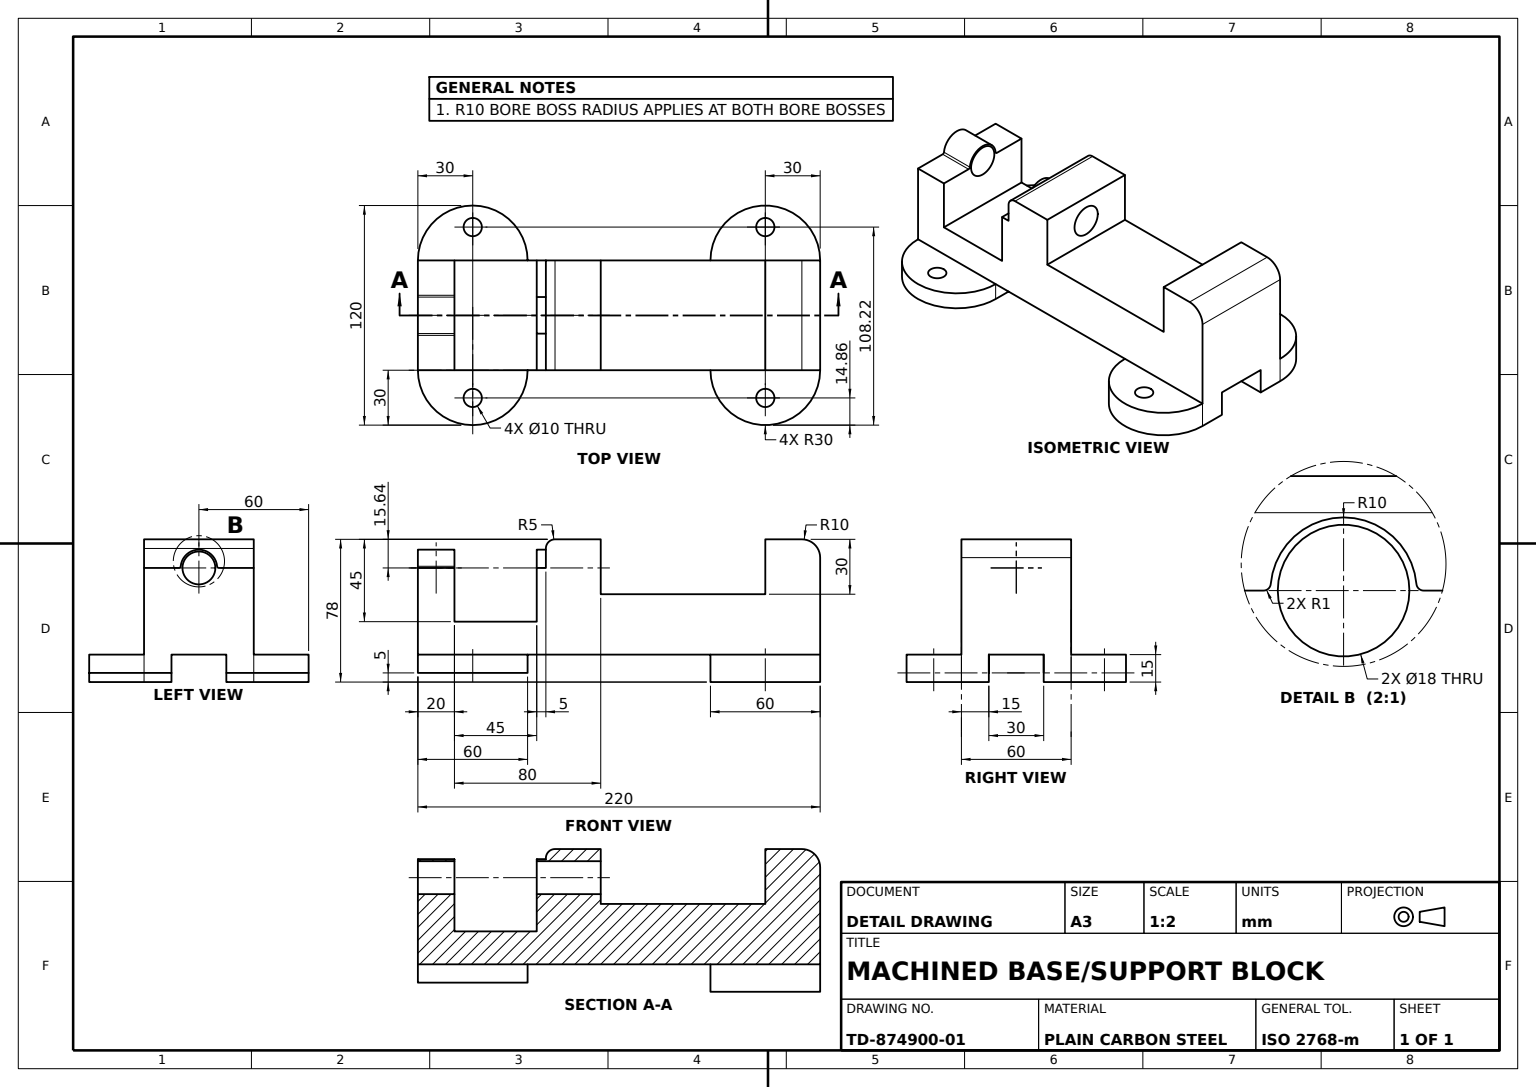
from build123d import *

# Parameters (mm, degrees)
BASE_PLATE_DEPTH           = 15
BODY_BLOCK_SKETCH_W        = 200
BODY_BLOCK_SKETCH_H        = 60
BODY_BLOCK_DEPTH           = 48
FIXED_JAW_SKETCH_W         = 60
FIXED_JAW_SKETCH_H         = 63
FIXED_JAW_DEPTH            = 20
GUIDE_CHANNEL_SKETCH_W     = 60
GUIDE_CHANNEL_SKETCH_H     = 60
GUIDE_CHANNEL_CUT_DEPTH    = 30
CHANNEL_END_CUT_SKETCH_W   = 30
CHANNEL_END_CUT_SKETCH_H   = 60
CHANNEL_END_CUT_DEPTH      = 30
JAW_SLOT_SKETCH_W          = 50
JAW_SLOT_SKETCH_H          = 60
JAW_SLOT_CUT_DEPTH         = 45
SLOT_RAIL_SKETCH_R         = 10
SLOT_RAIL_DEPTH            = 5
SCREW_BORE_SKETCH_R        = 9
SCREW_BORE_DEPTH           = 79
SCREW_POCKET_CUT_DEPTH     = 40
SCREW_BOSS_SKETCH_R        = 10
SCREW_BOSS_SKETCH_R_2      = 9
SCREW_BOSS_DEPTH           = 20
FIXED_JAW_FILLET_R10_R     = 10
JAW_SLOT_FILLET_R5_R       = 5
SCREW_BOSS_FILLET_R1_A_R   = 1
SCREW_BOSS_FILLET_R1_B_R   = 1
MOUNTING_FLANGE_SKETCH_W   = 60
MOUNTING_FLANGE_SKETCH_H   = 10
MOUNTING_FLANGE_DEPTH      = 30
FLANGE_RECESS_CUT_DEPTH    = 15
MOUNTING_LUG_SKETCH_W      = 60
MOUNTING_LUG_SKETCH_H      = 10
MOUNTING_LUG_DEPTH         = 15
REAR_JAW_BLOCK_SKETCH_W    = 60
REAR_JAW_BLOCK_SKETCH_H    = 15
REAR_JAW_BLOCK_DEPTH       = 30
REAR_JAW_CHANNEL_CUT_DEPTH = 30
REAR_JAW_NOTCH_CUT_DEPTH   = 30
REAR_LUG_SKETCH_W          = 60
REAR_LUG_SKETCH_H          = 15
REAR_LUG_DEPTH             = 15
LUG_CLEARANCE_CUT_SKETCH_R = 5
LUG_CLEARANCE_CUT_DEPTH    = 15


with BuildPart() as part:
    # Base Plate Sketch → Base Plate (new body)
    with BuildSketch(Plane(origin=(0, 0, 0), x_dir=(1, 0, 0), z_dir=(0, 1, 0))):
        Polygon((0, 0), (100, 0), (100, 60), (-100, 60), (-100, 0), align=None)
    extrude(amount=BASE_PLATE_DEPTH)

    # Body Block Sketch → Body Block (add)
    with BuildSketch(Plane(origin=(0, 15, 0), x_dir=(1, 0, 0), z_dir=(0, 1, 0))):
        with Locations((0, 30)):
            Rectangle(BODY_BLOCK_SKETCH_W, BODY_BLOCK_SKETCH_H)
    extrude(amount=BODY_BLOCK_DEPTH)

    # Fixed Jaw Sketch → Fixed Jaw (add)
    with BuildSketch(Plane(origin=(100, 0, 0), x_dir=(0, 0, -1), z_dir=(1, 0, 0))):
        with Locations((30, 31.5)):
            Rectangle(FIXED_JAW_SKETCH_W, FIXED_JAW_SKETCH_H)
    extrude(amount=FIXED_JAW_DEPTH)

    # Guide Channel Sketch → Guide Channel Cut (cut)
    with BuildSketch(Plane(origin=(0, 63, 0), x_dir=(1, 0, 0), z_dir=(0, 1, 0))):
        with Locations((60, 30)):
            Rectangle(GUIDE_CHANNEL_SKETCH_W, GUIDE_CHANNEL_SKETCH_H)
    extrude(amount=-GUIDE_CHANNEL_CUT_DEPTH, mode=Mode.SUBTRACT)

    # Channel End Cut Sketch → Channel End Cut (cut)
    with BuildSketch(Plane(origin=(0, 63, 0), x_dir=(1, 0, 0), z_dir=(0, 1, 0))):
        with Locations((15, 30)):
            Rectangle(CHANNEL_END_CUT_SKETCH_W, CHANNEL_END_CUT_SKETCH_H)
    extrude(amount=-CHANNEL_END_CUT_DEPTH, mode=Mode.SUBTRACT)

    # Jaw Slot Sketch → Jaw Slot Cut (cut)
    with BuildSketch(Plane(origin=(0, 63, 0), x_dir=(1, 0, 0), z_dir=(0, 1, 0))):
        with Locations((-55, 30)):
            Rectangle(JAW_SLOT_SKETCH_W, JAW_SLOT_SKETCH_H)
    extrude(amount=-JAW_SLOT_CUT_DEPTH, mode=Mode.SUBTRACT)

    # Slot Rail Sketch → Slot Rail (add)
    with BuildSketch(Plane.ZY.offset(30)):
        with Locations((-30, 47.357372748)):
            Circle(SLOT_RAIL_SKETCH_R)
        with BuildLine():
            Line((0, 18), (0, 47.357372748))
            Line((0, 47.357372748), (-20, 47.357372748))
            ThreePointArc((-20, 47.357372748), (-30, 37.357372748), (-40, 47.357372748))
            Line((-40, 47.357372748), (-60, 47.357372748))
            Line((-60, 47.357372748), (-60, 18))
            Line((-60, 18), (0, 18))
        make_face()
    extrude(amount=SLOT_RAIL_DEPTH)

    # Screw Bore Sketch → Screw Bore (cut, symmetric)
    with BuildSketch(Plane.ZY.offset(35)):
        with Locations((-30, 47.357372748)):
            Circle(SCREW_BORE_SKETCH_R)
    extrude(amount=SCREW_BORE_DEPTH, both=True, mode=Mode.SUBTRACT)

    # Screw Pocket Sketch → Screw Pocket Cut (cut)
    with BuildSketch(Plane.ZY.offset(100)):
        with BuildLine():
            ThreePointArc((-39, 47.357372748), (-30, 56.357372748), (-21, 47.357372748))
            Line((-21, 47.357372748), (0, 47.357372748))
            Line((0, 47.357372748), (0, 63))
            Line((0, 63), (-60, 63))
            Line((-60, 63), (-60, 47.357372748))
            Line((-60, 47.357372748), (-39, 47.357372748))
        make_face()
    extrude(amount=-SCREW_POCKET_CUT_DEPTH, mode=Mode.SUBTRACT)

    # Screw Boss Sketch → Screw Boss (add)
    with BuildSketch(Plane.ZY.offset(100)):
        with Locations((-30, 47.357372748)):
            Circle(SCREW_BOSS_SKETCH_R)
        with Locations(Location((-30, 47.357372748, 0), (0, 0, 180))):
            Circle(SCREW_BOSS_SKETCH_R_2, mode=Mode.SUBTRACT)
    extrude(amount=-SCREW_BOSS_DEPTH)

    # Fixed Jaw Fillet R10
    fixed_jaw_fillet_r10_edges = [part.edges().sort_by_distance(p)[0] for p in [
        (120, 63, -30),
    ]]
    fillet(fixed_jaw_fillet_r10_edges, radius=FIXED_JAW_FILLET_R10_R)

    # Jaw Slot Fillet R5
    jaw_slot_fillet_r5_edges = [part.edges().sort_by_distance(p)[0] for p in [
        (-30, 63, -30),
    ]]
    fillet(jaw_slot_fillet_r5_edges, radius=JAW_SLOT_FILLET_R5_R)

    # Screw Boss Fillet R1 A
    screw_boss_fillet_r1_a_edges = [part.edges().sort_by_distance(p)[0] for p in [
        (-90, 47.357372748, -20),
    ]]
    fillet(screw_boss_fillet_r1_a_edges, radius=SCREW_BOSS_FILLET_R1_A_R)

    # Screw Boss Fillet R1 B
    screw_boss_fillet_r1_b_edges = [part.edges().sort_by_distance(p)[0] for p in [
        (-90, 47.357372748, -40),
    ]]
    fillet(screw_boss_fillet_r1_b_edges, radius=SCREW_BOSS_FILLET_R1_B_R)



with BuildPart() as body_2:
    # Mounting Flange Sketch → Mounting Flange (new body)
    with BuildSketch(Plane.XY):
        with Locations((-70, -5)):
            Rectangle(MOUNTING_FLANGE_SKETCH_W, MOUNTING_FLANGE_SKETCH_H)
    extrude(amount=MOUNTING_FLANGE_DEPTH)

    # Flange Recess Sketch → Flange Recess Cut (cut)
    with BuildSketch(Plane(origin=(0, 0, 0), x_dir=(1, 0, 0), z_dir=(0, 1, 0))):
        with BuildLine():
            Line((-40, -30), (-40, 0))
            ThreePointArc((-40, 0), (-48.786796564, -21.213203436), (-70, -30))
            Line((-70, -30), (-40, -30))
        make_face()
        with BuildLine():
            Line((-100, -30), (-70, -30))
            ThreePointArc((-70, -30), (-91.213203436, -21.213203436), (-100, 0))
            Line((-100, 0), (-100, -30))
        make_face()
    extrude(amount=-FLANGE_RECESS_CUT_DEPTH, mode=Mode.SUBTRACT)


with BuildPart() as part_1:
    add(part.part)

    add(body_2.part)  # Mounting Lug merges body 2
    # Mounting Lug Sketch → Mounting Lug (add)
    with BuildSketch(Plane(origin=(0, 0, 0), x_dir=(-1, 0, 0), z_dir=(0, 0, -1))):
        with Locations((70, -5)):
            Rectangle(MOUNTING_LUG_SKETCH_W, MOUNTING_LUG_SKETCH_H)
    extrude(amount=MOUNTING_LUG_DEPTH)

    # Mounting Lug Mirror: part across plane


with BuildPart() as part_2:
    add(part_1.part)
    add(part_1.part.mirror(Plane.XY.offset(-30)))



with BuildPart() as body_2_2:
    # Rear Jaw Block Sketch → Rear Jaw Block (new body)
    with BuildSketch(Plane.XY):
        with Locations((90, -7.5)):
            Rectangle(REAR_JAW_BLOCK_SKETCH_W, REAR_JAW_BLOCK_SKETCH_H)
    extrude(amount=REAR_JAW_BLOCK_DEPTH)

    # Rear Jaw Channel Sketch → Rear Jaw Channel Cut (cut)
    with BuildSketch(Plane(origin=(0, 0, 0), x_dir=(1, 0, 0), z_dir=(0, 1, 0))):
        with BuildLine():
            ThreePointArc((90, -30), (68.786796564, -21.213203436), (60, 0))
            Line((60, 0), (60, -30))
            Line((60, -30), (90, -30))
        make_face()
    extrude(amount=-REAR_JAW_CHANNEL_CUT_DEPTH, mode=Mode.SUBTRACT)

    # Rear Jaw Notch Sketch → Rear Jaw Notch Cut (cut)
    with BuildSketch(Plane(origin=(0, 0, 0), x_dir=(1, 0, 0), z_dir=(0, 1, 0))):
        with BuildLine():
            Line((120, -30), (120, 0))
            ThreePointArc((120, 0), (111.213203436, -21.213203436), (90, -30))
            Line((90, -30), (120, -30))
        make_face()
    extrude(amount=-REAR_JAW_NOTCH_CUT_DEPTH, mode=Mode.SUBTRACT)


with BuildPart() as part_3:
    add(part_2.part)

    add(body_2_2.part)  # Rear Lug merges body 2 2
    # Rear Lug Sketch → Rear Lug (add)
    with BuildSketch(Plane(origin=(0, 0, 0), x_dir=(-1, 0, 0), z_dir=(0, 0, -1))):
        with Locations((-90, -7.5)):
            Rectangle(REAR_LUG_SKETCH_W, REAR_LUG_SKETCH_H)
    extrude(amount=REAR_LUG_DEPTH)

    # Rear Lug Mirror: part across plane


with BuildPart() as part_4:
    add(part_3.part)
    add(part_3.part.mirror(Plane.XY.offset(-30)))

    # Lug Clearance Cut Sketch → Lug Clearance Cut (cut)
    with BuildSketch(Plane(origin=(0, 0, 0), x_dir=(1, 0, 0), z_dir=(0, 1, 0))):
        with Locations(Location((-70, -15.138677931, 0), (0, 0, 270))):
            Circle(LUG_CLEARANCE_CUT_SKETCH_R)
        with Locations(Location((90, -15.138677931, 0), (0, 0, 270))):
            Circle(LUG_CLEARANCE_CUT_SKETCH_R)
        with Locations(Location((-70, 78.223643899, 0), (0, 0, 270))):
            Circle(LUG_CLEARANCE_CUT_SKETCH_R)
        with Locations(Location((90, 78.223643899, 0), (0, 0, 270))):
            Circle(LUG_CLEARANCE_CUT_SKETCH_R)
    extrude(amount=-LUG_CLEARANCE_CUT_DEPTH, mode=Mode.SUBTRACT)


solid = part_4.part
